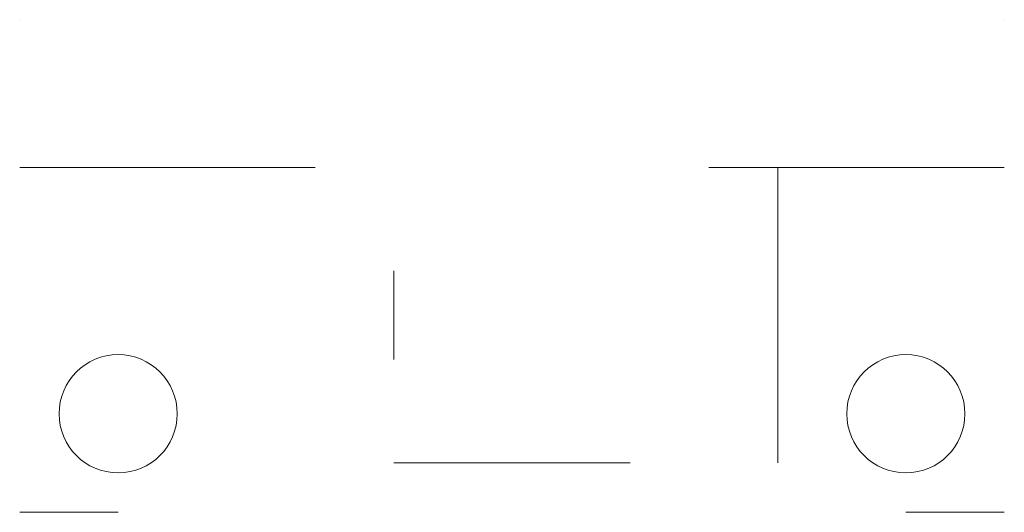
# Model space of a CAD drawing. Units: inches. Extents: x 102.2 to 202.2, y 97.8 to 147.8.
import ezdxf

# ---------------------------------------------------------------- set-up
doc = ezdxf.new("R2010")
doc.units = ezdxf.units.IN
doc.header["$MEASUREMENT"] = 0
doc.layers.add('M-CONS', color=8, linetype='Continuous', lineweight=13)

msp = doc.modelspace()

# ---------------------------------------------------------------- linework, layer by layer
at = {"layer": 'M-CONS'}
for p, q in [((102.16, 147.81, 15), (102.16, 147.81, 45)), ((202.16, 147.81), (202.16, 147.81, 45)), ((179.16, 102.81, 15), (179.16, 132.81, 15)), ((102.16, 97.81, 15), (112.16, 97.81, 15))]:
    msp.add_line(p, q, dxfattribs=at)
at = {"layer": 'M-CONS', "extrusion": (0, -1, 0)}
for p, q in [((132.16, 132.81, 45), (102.16, 132.81, 45)), ((202.16, 132.81, 45), (172.16, 132.81, 45)), ((202.16, 132.81, 45), (172.16, 132.81, 45))]:
    msp.add_line(p, q, dxfattribs=at)
at = {"layer": 'M-CONS', "extrusion": (1, 0, 0)}
msp.add_line((202.16, 97.81, 15), (192.16, 97.81, 15), dxfattribs=at)
at = {"layer": 'M-CONS', "extrusion": (0, -1, 0), "elevation": -102.81}
msp.add_lwpolyline([(140.16, 45, 1), (164.16, 45)], format="xyb", close=True, dxfattribs=at)
at = {"layer": 'M-CONS', "extrusion": (1, 0, 0)}
for centre in [(117.81, 50, 140.16), (117.81, 50, 179.16)]:
    msp.add_circle(centre, 4.5, dxfattribs=at)
at = {"layer": 'M-CONS'}
for centre in [(112.16, 107.81, 15), (192.16, 107.81, 15)]:
    msp.add_circle(centre, 6, dxfattribs=at)

doc.saveas('drawing.dxf')
